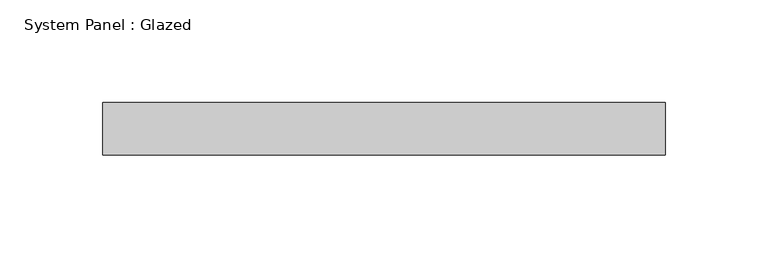
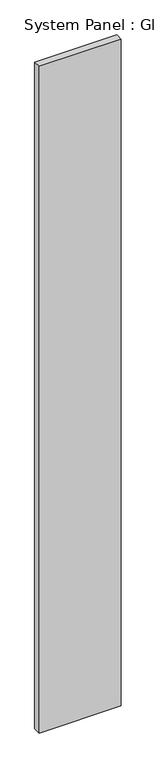
"""IFC4 building model written with IfcOpenShell, lengths in millimetres: plate geometry, System Panel : Glazed."""

from ifc_helpers import new_model, si_unit, origin, origin_with_axes, place, context, project, spatial, polyline, outline, extrude, source, transform, mapped, element, save


def system_panel_glazed_a1694ec4(model_context):
    return source(origin(), model_context, "Body", "SweptSolid", [
        extrude(outline(polyline([(136.525, -44.45), (-136.525, -44.45), (-136.525, -19.05), (136.525, -19.05), (136.525, -44.45)])), origin_with_axes(), (0.0, 0.0, 1.0), 2343.15),
    ])


if __name__ == "__main__":
    model = new_model("IFC4")
    model_context = context("Model", 3, world=origin())
    ifc_project = project(units=[si_unit("LENGTHUNIT", "METRE", prefix="MILLI")], contexts=[model_context])
    site = spatial("IfcSite", under=ifc_project)
    building = spatial("IfcBuilding", under=site)
    placement = place(None, origin())
    system_panel_glazed_shape = system_panel_glazed_a1694ec4(model_context)
    element("IfcPlate", 1, ObjectType="System Panel : Glazed", at=placement, inside=building, context=model_context, shape_type="MappedRepresentation", body=[
        mapped(system_panel_glazed_shape, transform((0.0, 0.0, 0.0), x_axis=(1.0, 0.0, 0.0), y_axis=(0.0, 1.0, 0.0), z_axis=(0.0, 0.0, 1.0))),
    ])
    save(model, "model.ifc")

# Revit data of these elements
# Type "System Panel : Glazed"
#   Construction Type Id = "GSP4R"
#   Analytic Construction = "1/8 in Pilkington single glazing"
#   Visual Light Transmittance = 0.9
#   Solar Heat Gain Coefficient = 0.86
#   Heat Transfer Coefficient (U) = 1.18115 BTU/(h·ft²·°F)
# Element 1 (IfcPlate, "System Panel : Glazed")
#   Materials on its faces: "Glass"
# Materials
#   "Glass": class "Glass", colour RGB 0 128 192, transparency 0.75, Description = "Soda Lime Glass", Cost = 0
